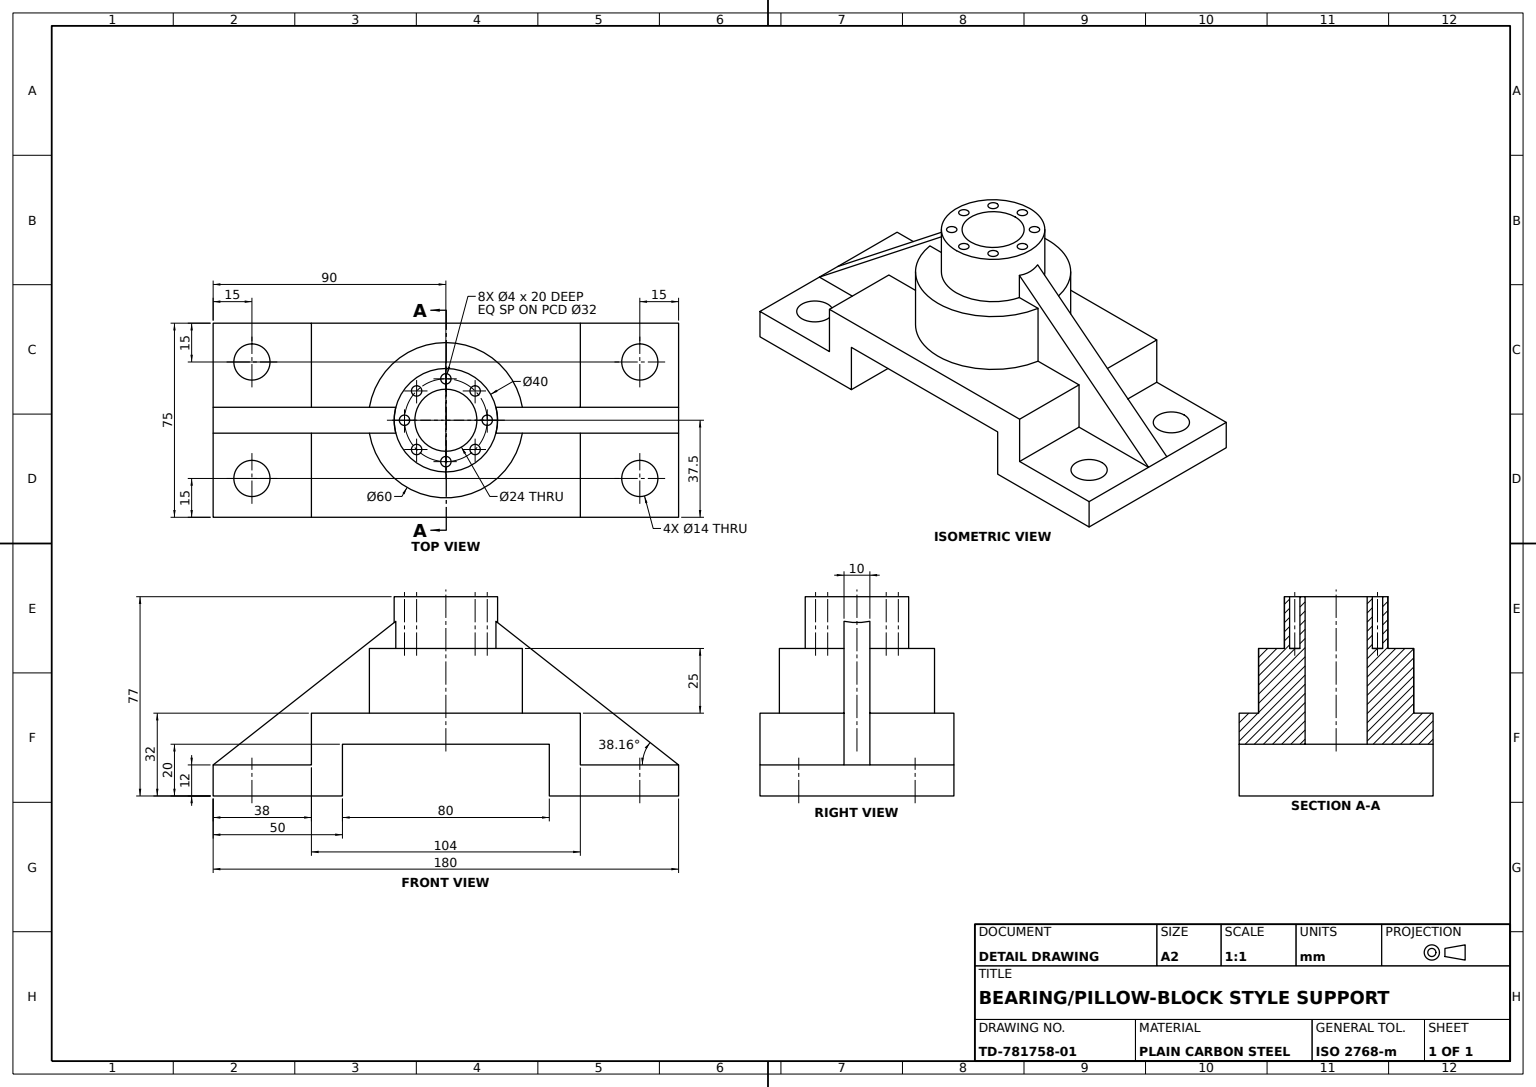
from build123d import *

# Parameters (mm, degrees)
BASE_PLATE_DEPTH              = 75
BOSS_60_SKETCH_R              = 30
BOSS_60_DEPTH                 = 25
HUB_40_SKETCH_R               = 20
HUB_40_DEPTH                  = 20
BOLT_CIRCLE_8X_4_SKETCH_R     = 2
BOLT_CIRCLE_HOLES_8X_4_DEPTH  = 20
BORE_24_SKETCH_R              = 12
BORE_24_DEPTH                 = 210.652092763
MOUNTING_HOLES_4X_14_SKETCH_R = 7
MOUNTING_HOLES_4X_14_DEPTH    = 20
REINFORCING_RIB_A_REACH       = 201.337
RIB_A_SKETCH_WALL_W           = 489.696521402
RIB_A_SKETCH_WALL_H           = 10
REINFORCING_RIB_B_REACH       = 201.337
RIB_B_SKETCH_WALL_W           = 489.696521402
RIB_B_SKETCH_WALL_H           = 10


with BuildPart() as part:
    # Base Plate Profile → Base Plate (new body)
    with BuildSketch(Plane.XY):
        Polygon((0, 0), (50, 0), (50, 20), (130, 20), (130, 0), (180, 0), (180, 12), (142, 12), (142, 32), (38, 32), (38, 12), (0, 12), align=None)
    extrude(amount=-BASE_PLATE_DEPTH)

    # Boss Ø60 Sketch → Boss Ø60 (add)
    with BuildSketch(Plane(origin=(0, 32, 0), x_dir=(1, 0, 0), z_dir=(0, 1, 0))):
        with Locations(Location((90, 37.5, 0), (0, 0, 270))):
            Circle(BOSS_60_SKETCH_R)
    extrude(amount=BOSS_60_DEPTH)

    # Hub Ø40 Sketch → Hub Ø40 (add)
    with BuildSketch(Plane(origin=(0, 57, 0), x_dir=(1, 0, 0), z_dir=(0, 1, 0))):
        with Locations(Location((90, 37.5, 0), (0, 0, 270))):
            Circle(HUB_40_SKETCH_R)
    extrude(amount=HUB_40_DEPTH)

    # Bolt Circle 8xØ4 Sketch → Bolt Circle Holes 8xØ4 (cut)
    with BuildSketch(Plane(origin=(0, 77, 0), x_dir=(1, 0, 0), z_dir=(0, 1, 0))):
        with Locations(Location((90, 53.5, 0), (0, 0, 270))):
            Circle(BOLT_CIRCLE_8X_4_SKETCH_R)
        with Locations(Location((101.313708499, 48.813708499, 0), (0, 0, 270))):
            Circle(BOLT_CIRCLE_8X_4_SKETCH_R)
        with Locations(Location((106, 37.5, 0), (0, 0, 270))):
            Circle(BOLT_CIRCLE_8X_4_SKETCH_R)
        with Locations(Location((101.313708499, 26.186291501, 0), (0, 0, 270))):
            Circle(BOLT_CIRCLE_8X_4_SKETCH_R)
        with Locations(Location((90, 21.5, 0), (0, 0, 270))):
            Circle(BOLT_CIRCLE_8X_4_SKETCH_R)
        with Locations(Location((78.686291501, 26.186291501, 0), (0, 0, 270))):
            Circle(BOLT_CIRCLE_8X_4_SKETCH_R)
        with Locations(Location((74, 37.5, 0), (0, 0, 270))):
            Circle(BOLT_CIRCLE_8X_4_SKETCH_R)
        with Locations(Location((78.686291501, 48.813708499, 0), (0, 0, 270))):
            Circle(BOLT_CIRCLE_8X_4_SKETCH_R)
    extrude(amount=-BOLT_CIRCLE_HOLES_8X_4_DEPTH, mode=Mode.SUBTRACT)

    # Bore Ø24 Sketch → Bore Ø24 (cut, through all)
    with BuildSketch(Plane(origin=(0, 77, 0), x_dir=(1, 0, 0), z_dir=(0, 1, 0))):
        with Locations(Location((90, 37.5, 0), (0, 0, 270))):
            Circle(BORE_24_SKETCH_R)
    extrude(amount=-BORE_24_DEPTH, mode=Mode.SUBTRACT)

    # Mounting Holes 4xØ14 Sketch → Mounting Holes 4xØ14 (cut)
    with BuildSketch(Plane(origin=(0, 12, 0), x_dir=(1, 0, 0), z_dir=(0, 1, 0))):
        with Locations(Location((165, 60, 0), (0, 0, 270))):
            Circle(MOUNTING_HOLES_4X_14_SKETCH_R)
        with Locations(Location((165, 15, 0), (0, 0, 270))):
            Circle(MOUNTING_HOLES_4X_14_SKETCH_R)
        with Locations(Location((15, 60, 0), (0, 0, 270))):
            Circle(MOUNTING_HOLES_4X_14_SKETCH_R)
        with Locations(Location((15, 15, 0), (0, 0, 270))):
            Circle(MOUNTING_HOLES_4X_14_SKETCH_R)
    extrude(amount=-MOUNTING_HOLES_4X_14_DEPTH, mode=Mode.SUBTRACT)

    # Rib A Sketch wall → Reinforcing Rib A (add, up to next)
    with BuildSketch(Plane(origin=(145, 39.5, -37.5), x_dir=(0.786318338822, -0.617821551932, 0), z_dir=(0.617821551932, 0.786318338822, 0)), mode=Mode.PRIVATE) as reinforcing_rib_a_sk1:
        Rectangle(RIB_A_SKETCH_WALL_W, RIB_A_SKETCH_WALL_H)
    reinforcing_rib_a_tool1 = extrude(reinforcing_rib_a_sk1.sketch, amount=-REINFORCING_RIB_A_REACH, mode=Mode.PRIVATE) - part.part
    add(reinforcing_rib_a_tool1.solids().sort_by_distance((145, 39.5, -37.5))[0])

    # Rib B Sketch wall → Reinforcing Rib B (add, up to next)
    with BuildSketch(Plane(origin=(35, 39.5, -37.5), x_dir=(-0.786318338822, -0.617821551932, 0), z_dir=(0.617821551932, -0.786318338822, 0)), mode=Mode.PRIVATE) as reinforcing_rib_b_sk1:
        Rectangle(RIB_B_SKETCH_WALL_W, RIB_B_SKETCH_WALL_H)
    reinforcing_rib_b_tool1 = extrude(reinforcing_rib_b_sk1.sketch, amount=REINFORCING_RIB_B_REACH, mode=Mode.PRIVATE) - part.part
    add(reinforcing_rib_b_tool1.solids().sort_by_distance((35, 39.5, -37.5))[0])


solid = part.part
